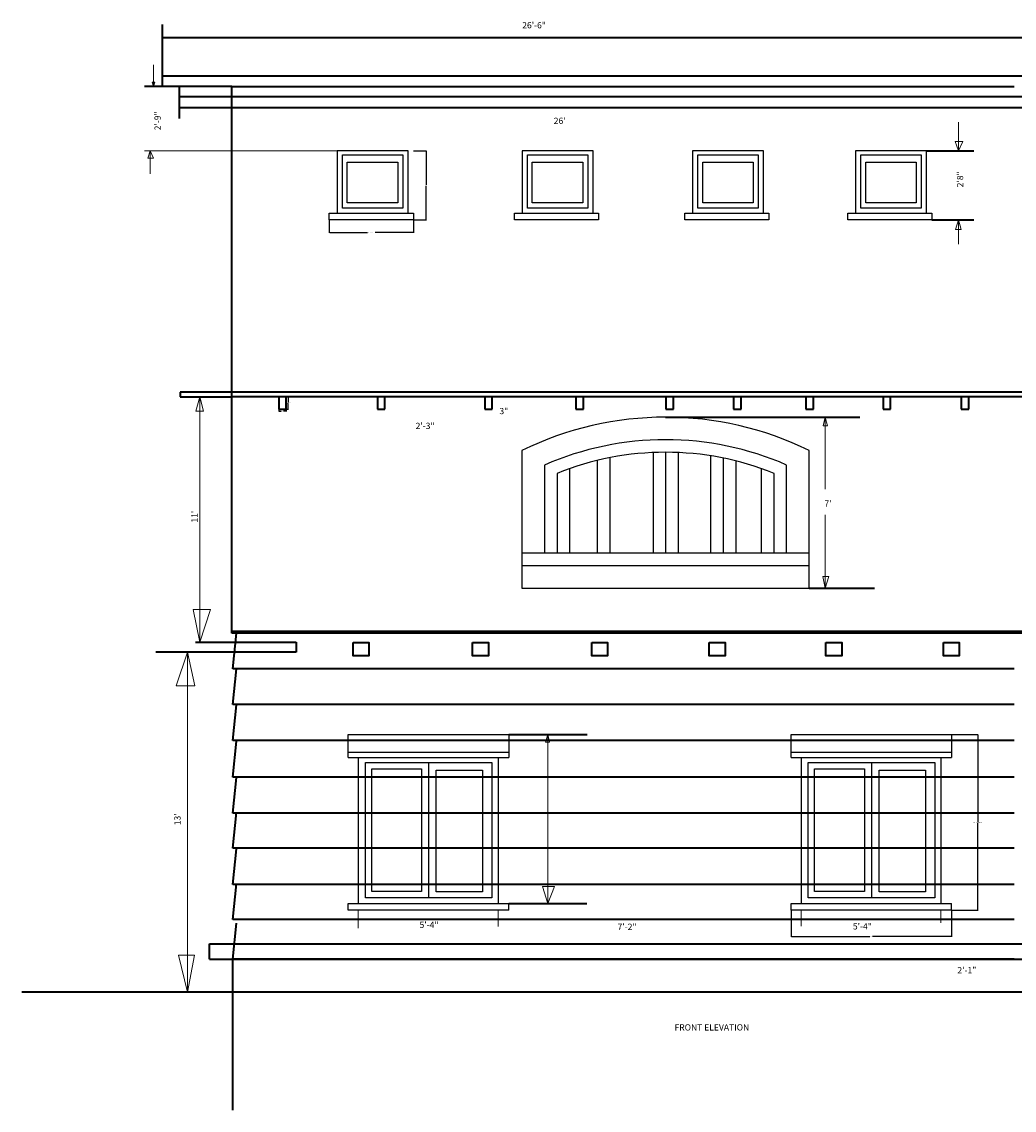
# Model space of a CAD drawing. Units: inches. Extents: x 2633 to 3277, y 1081 to 1518.
# Tile 1 of 2: x 2633 to 3029, y 1081 to 1515. Entities that reach past the tile are written whole.
import ezdxf

# ---------------------------------------------------------------- set-up
doc = ezdxf.new("R2010")
doc.units = ezdxf.units.IN
for name, color, linetype, lineweight in [('A-ANNO-DIMS', 2, 'Continuous', 18), ('A-ANNO-TEXT', 7, 'Continuous', 18), ('A-ELEV', 7, 'Continuous', 35), ('A-GLAZ', 4, 'Continuous', 25)]:
    doc.layers.add(name, color=color, linetype=linetype, lineweight=lineweight)
doc.styles.get("Standard").update_dxf_attribs({"font": 'arial.ttf'})
doc.dimstyles.get("Standard").update_dxf_attribs({"dimtxt": 0.18, "dimasz": 0.18, "dimexe": 0.18, "dimexo": 0.0625, "dimgap": 0.09, "dimtad": 0, "dimtih": 1, "dimtoh": 1, "dimdec": 4, "dimzin": 0, "dimdsep": 46, "dimtxsty": 'Standard', "dimcen": 0.09, "dimadec": 0, "dimazin": 0, "dimtfac": 1, "dimtdec": 4, "dimtofl": 0, "dimtmove": 0, "dimatfit": 3, "dimfxl": 1, "dimtolj": 1, "dimtzin": 0, "dimarcsym": 0})

# ---------------------------------------------------------------- blocks, each defined once
blk = doc.blocks.new('WIN-SMALL')
for points in [[(2758.75, 1438.68), (2787.06, 1438.68), (2787.06, 1463.6), (2758.75, 1463.6)], [(2760.89, 1461.89), (2784.92, 1461.89), (2784.92, 1440.71), (2760.89, 1440.71)], [(2762.78, 1458.97), (2782.94, 1458.97), (2782.94, 1442.85), (2762.78, 1442.85)], [(2755.63, 1438.68), (2789.18, 1438.68), (2789.18, 1436.03), (2755.63, 1436.03)]]:
    blk.add_lwpolyline(points, close=True)
blk = doc.blocks.new('WIN-1600-DBL')
for p, q in [((2763.18, 1221.7), (2763.18, 1230.77)), ((2763.18, 1230.77), (2827.18, 1230.77)), ((2827.18, 1230.77), (2827.18, 1221.7)), ((2763.18, 1223.71), (2827.18, 1223.77)), ((2763.18, 1221.7), (2827.18, 1221.7)), ((2767.18, 1221.7), (2767.18, 1163.47)), ((2822.92, 1221.7), (2822.92, 1163.47)), ((2795.24, 1219.61), (2795.24, 1165.66)), ((2763.18, 1160.77), (2763.18, 1163.47)), ((2763.18, 1163.47), (2827.18, 1163.47)), ((2827.18, 1160.77), (2827.18, 1163.47)), ((2827.18, 1160.77), (2763.18, 1160.77))]:
    blk.add_line(p, q)
for points in [[(2770, 1219.61), (2820.48, 1219.61), (2820.48, 1165.66), (2770, 1165.66)], [(2772.55, 1217.06), (2792.42, 1217.06), (2792.42, 1168.21), (2772.55, 1168.21)], [(2798.27, 1216.53), (2816.76, 1216.53), (2816.76, 1168.1), (2798.27, 1168.1)]]:
    blk.add_lwpolyline(points, close=True)
blk = doc.blocks.new('CORBEL-A')
for p, q in [((0, 4.96), (0, 0)), ((3, 0), (3, 4.96)), ((0, 0), (3, 0))]:
    blk.add_line(p, q)
blk = doc.blocks.new('*D6')
at = {"layer": 'A-ANNO-DIMS', "color": 0, "lineweight": -2, "transparency": 16777216}
for p, q in [((2755.63, 1435.97), (2755.63, 1430.82)), ((2789.18, 1435.97), (2789.18, 1430.82)), ((2755.81, 1431), (2770.84, 1431)), ((2789, 1431), (2773.97, 1431))]:
    blk.add_line(p, q, dxfattribs=at)
at = {"layer": 'A-ANNO-DIMS', "color": 0, "transparency": 16777216}
for points in [[(2755.81, 1431.03), (2755.81, 1430.97), (2755.63, 1431)], [(2789, 1431.03), (2789, 1430.97), (2789.18, 1431)]]:
    blk.add_solid(points, dxfattribs=at)
at = {"layer": 'Defpoints', "color": 0, "transparency": 16777216}
for p in [(2755.63, 1436.03), (2789.18, 1436.03), (2789.18, 1431)]:
    blk.add_point(p, dxfattribs=at)
at = {"layer": 'A-ANNO-DIMS', "color": 0, "transparency": 16777216, "insert": (2772.4, 1431), "char_height": 0.18, "attachment_point": 5}
blk.add_mtext('\\A1;SMALL WINDOW 34 TYP.', dxfattribs=at)
blk = doc.blocks.new('*D7')
at = {"layer": 'A-ANNO-DIMS', "color": 0, "lineweight": -2, "transparency": 16777216}
for p, q in [((2789.24, 1463.6), (2794.39, 1463.6)), ((2794.21, 1463.42), (2794.21, 1450)), ((2794.21, 1436.21), (2794.21, 1449.64)), ((2789.24, 1436.03), (2794.39, 1436.03))]:
    blk.add_line(p, q, dxfattribs=at)
at = {"layer": 'A-ANNO-DIMS', "color": 0, "transparency": 16777216}
for points in [[(2794.18, 1463.42), (2794.24, 1463.42), (2794.21, 1463.6)], [(2794.18, 1436.21), (2794.24, 1436.21), (2794.21, 1436.03)]]:
    blk.add_solid(points, dxfattribs=at)
at = {"layer": 'Defpoints', "color": 0, "transparency": 16777216}
for p in [(2789.18, 1463.6), (2794.21, 1463.6), (2789.18, 1436.03)]:
    blk.add_point(p, dxfattribs=at)
at = {"layer": 'A-ANNO-DIMS', "color": 0, "transparency": 16777216, "insert": (2794.21, 1449.82), "char_height": 0.18, "attachment_point": 5}
blk.add_mtext('\\A1;28 TYP.', dxfattribs=at)
blk = doc.blocks.new('*D8')
at = {"layer": 'A-ANNO-DIMS', "color": 0, "lineweight": -2, "transparency": 16777216}
for p, q in [((3003.8, 1230.77), (3014.41, 1230.77)), ((3014.23, 1230.59), (3014.23, 1195.96)), ((3014.23, 1160.95), (3014.23, 1195.59)), ((3003.8, 1160.77), (3014.41, 1160.77))]:
    blk.add_line(p, q, dxfattribs=at)
at = {"layer": 'A-ANNO-DIMS', "color": 0, "transparency": 16777216}
for points in [[(3014.2, 1230.59), (3014.26, 1230.59), (3014.23, 1230.77)], [(3014.2, 1160.95), (3014.26, 1160.95), (3014.23, 1160.77)]]:
    blk.add_solid(points, dxfattribs=at)
at = {"layer": 'Defpoints', "color": 0, "transparency": 16777216}
for p in [(3003.73, 1230.77), (3014.23, 1230.77), (3003.73, 1160.77)]:
    blk.add_point(p, dxfattribs=at)
at = {"layer": 'A-ANNO-DIMS', "color": 0, "transparency": 16777216, "insert": (3014.23, 1195.77), "char_height": 0.18, "attachment_point": 5}
blk.add_mtext('\\A1;DOUBLE WINDOW 1600 70 TYP.', dxfattribs=at)
blk = doc.blocks.new('*D9')
at = {"layer": 'A-ANNO-DIMS', "color": 0, "lineweight": -2, "transparency": 16777216}
for p, q in [((2939.73, 1160.71), (2939.73, 1150.09)), ((3003.73, 1160.71), (3003.73, 1150.09)), ((2939.91, 1150.27), (2971.21, 1150.27)), ((3003.55, 1150.27), (2972.26, 1150.27))]:
    blk.add_line(p, q, dxfattribs=at)
at = {"layer": 'A-ANNO-DIMS', "color": 0, "transparency": 16777216}
for points in [[(2939.91, 1150.3), (2939.91, 1150.24), (2939.73, 1150.27)], [(3003.55, 1150.3), (3003.55, 1150.24), (3003.73, 1150.27)]]:
    blk.add_solid(points, dxfattribs=at)
at = {"layer": 'Defpoints', "color": 0, "transparency": 16777216}
for p in [(2939.73, 1160.77), (3003.73, 1160.77), (3003.73, 1150.27)]:
    blk.add_point(p, dxfattribs=at)
at = {"layer": 'A-ANNO-DIMS', "color": 0, "transparency": 16777216, "insert": (2971.73, 1150.27), "char_height": 0.18, "attachment_point": 5}
blk.add_mtext('\\A1;64 TYP.', dxfattribs=at)
blk = doc.blocks.new('*D12')
at = {"layer": 'A-ANNO-DIMS', "color": 0, "lineweight": -2, "transparency": 16777216}
for p, q in [((2738.5, 1365.48), (2739.37, 1365.48)), ((2739.19, 1365.3), (2739.19, 1363.18)), ((2738.5, 1360.52), (2739.37, 1360.52)), ((2739.19, 1360.7), (2739.19, 1362.81))]:
    blk.add_line(p, q, dxfattribs=at)
at = {"layer": 'A-ANNO-DIMS', "color": 0, "transparency": 16777216}
for points in [[(2739.16, 1365.3), (2739.22, 1365.3), (2739.19, 1365.48)], [(2739.16, 1360.7), (2739.22, 1360.7), (2739.19, 1360.52)]]:
    blk.add_solid(points, dxfattribs=at)
at = {"layer": 'Defpoints', "color": 0, "transparency": 16777216}
for p in [(2738.44, 1365.48), (2739.19, 1365.48), (2738.44, 1360.52)]:
    blk.add_point(p, dxfattribs=at)
at = {"layer": 'A-ANNO-DIMS', "color": 0, "transparency": 16777216, "insert": (2739.19, 1363), "char_height": 0.18, "attachment_point": 5}
blk.add_mtext('\\A1;CORBEL A 5 TYP.', dxfattribs=at)
blk = doc.blocks.new('*D13')
at = {"layer": 'A-ANNO-DIMS', "color": 0, "lineweight": -2, "transparency": 16777216}
for p, q in [((2735.44, 1360.45), (2735.44, 1359.59)), ((2735.62, 1359.77), (2736.48, 1359.77)), ((2738.26, 1359.77), (2737.4, 1359.77)), ((2738.44, 1360.45), (2738.44, 1359.59))]:
    blk.add_line(p, q, dxfattribs=at)
at = {"layer": 'A-ANNO-DIMS', "color": 0, "transparency": 16777216}
for points in [[(2735.62, 1359.8), (2735.62, 1359.74), (2735.44, 1359.77)], [(2738.26, 1359.8), (2738.26, 1359.74), (2738.44, 1359.77)]]:
    blk.add_solid(points, dxfattribs=at)
at = {"layer": 'Defpoints', "color": 0, "transparency": 16777216}
for p in [(2735.44, 1360.52), (2738.44, 1360.52), (2738.44, 1359.77)]:
    blk.add_point(p, dxfattribs=at)
at = {"layer": 'A-ANNO-DIMS', "color": 0, "transparency": 16777216, "insert": (2736.94, 1359.77), "char_height": 0.18, "attachment_point": 5}
blk.add_mtext('\\A1;3 TYP.', dxfattribs=at)

msp = doc.modelspace()

# ---------------------------------------------------------------- linework, layer by layer
at = {"layer": 'A-ANNO-DIMS'}
for p, q in [((2685.55, 1489.27), (2685.55, 1497.82)), ((2685.55, 1489.27), (2685.05, 1490.87)), ((2685.05, 1490.87), (2686.02, 1490.87)), ((2686.02, 1490.87), (2685.55, 1489.27)), ((3006.52, 1463.6), (3006.52, 1474.98)), ((3006.52, 1463.6), (3005.21, 1467.22)), ((3005.21, 1467.22), (3008.18, 1467.22)), ((3008.18, 1467.22), (3006.52, 1463.6)), ((2684.17, 1463.6), (2682, 1463.6)), ((2684.17, 1463.6), (2683.31, 1460.56)), ((2758.75, 1463.6), (2684.17, 1463.6)), ((2684.17, 1463.6), (2684.17, 1454.36)), ((2685.55, 1460.56), (2684.17, 1463.6)), ((2683.31, 1460.56), (2685.55, 1460.56)), ((3006.52, 1436.03), (3005.33, 1432.15)), ((3006.52, 1436.03), (3006.52, 1426.33)), ((3007.59, 1432.15), (3006.52, 1436.03)), ((3005.33, 1432.15), (3007.59, 1432.15)), ((2704.03, 1365.48), (2702.38, 1359.8)), ((2704.03, 1365.48), (2704.03, 1267.58)), ((2705.46, 1359.8), (2704.03, 1365.48)), ((2702.38, 1359.8), (2705.46, 1359.8)), ((2953.34, 1357.35), (2952.57, 1353.88)), ((2953.34, 1357.35), (2953.34, 1328.63)), ((2954.23, 1353.88), (2953.34, 1357.35)), ((2952.57, 1353.88), (2954.23, 1353.88)), ((2953.34, 1318.37), (2953.34, 1289.2)), ((2953.34, 1289.2), (2952.42, 1293.75)), ((2952.42, 1293.75), (2954.75, 1293.75)), ((2954.75, 1293.75), (2953.34, 1289.2)), ((2704.03, 1267.58), (2701.36, 1280.64)), ((2701.36, 1280.64), (2708.25, 1280.64)), ((2708.25, 1280.64), (2704.03, 1267.58)), ((2699.04, 1263.58), (2694.62, 1250.15)), ((2699.04, 1263.58), (2699.04, 1128.1)), ((2702.02, 1250.15), (2699.04, 1263.58)), ((2694.62, 1250.15), (2702.02, 1250.15)), ((2842.72, 1230.77), (2841.86, 1227.77)), ((2842.72, 1163.47), (2842.72, 1230.77)), ((2843.41, 1227.77), (2842.72, 1230.77)), ((2841.86, 1227.77), (2843.41, 1227.77)), ((2842.72, 1163.47), (2840.59, 1170.21)), ((2840.59, 1170.21), (2845.42, 1170.21)), ((2845.42, 1170.21), (2842.72, 1163.47)), ((2767.18, 1160.77), (2767.18, 1153.52)), ((2822.92, 1160.77), (2822.92, 1154.28)), ((2943.73, 1160.77), (2943.73, 1154.35)), ((2999.47, 1160.77), (2999.47, 1155.65)), ((2699.04, 1128.1), (2695.5, 1142.8)), ((2695.5, 1142.8), (2701.93, 1142.8)), ((2701.93, 1142.8), (2699.04, 1128.1))]:
    msp.add_line(p, q, dxfattribs=at)
at = {"layer": 'A-ELEV'}
for p, q in [((2689.1, 1493.43), (2689.1, 1513.93)), ((2689.1, 1508.71), (3038.3, 1508.71)), ((2689.1, 1489.27), (2689.1, 1493.43)), ((2689.1, 1493.43), (3038.3, 1493.43)), ((2689.1, 1489.27), (2682, 1489.27)), ((2716.73, 1489.27), (2689.1, 1489.27)), ((2695.73, 1489.27), (2695.73, 1485.17)), ((2716.73, 1403.27), (2716.73, 1489.27)), ((2716.73, 1489.27), (3028.73, 1489.27)), ((2695.73, 1485.17), (3034.63, 1485.17)), ((2695.73, 1485.17), (2695.73, 1476.45)), ((2695.73, 1480.81), (3034.63, 1480.81)), ((2993.79, 1463.6), (3012.64, 1463.6)), ((2995.9, 1436.03), (3012.64, 1436.03)), ((2716.73, 1271.27), (2716.73, 1403.27)), ((2716.73, 1367.27), (2696.18, 1367.27)), ((2696.18, 1367.27), (2696.18, 1365.48)), ((2852.9, 1367.27), (2716.73, 1367.27)), ((3213.81, 1367.27), (2852.9, 1367.27)), ((2696.18, 1365.48), (2716.73, 1365.48)), ((2840.38, 1365.48), (2716.73, 1365.48)), ((3199.77, 1365.48), (2840.38, 1365.48)), ((2916.84, 1365.48), (2916.84, 1360.52)), ((2916.84, 1365.48), (2916.84, 1360.52)), ((2916.84, 1365.48), (2916.84, 1360.52)), ((2919.84, 1360.52), (2919.84, 1365.48)), ((2919.84, 1360.52), (2919.84, 1365.48)), ((2919.84, 1360.52), (2919.84, 1365.48)), ((2916.84, 1360.52), (2919.84, 1360.52)), ((2916.84, 1360.52), (2919.84, 1360.52)), ((2916.84, 1360.52), (2919.84, 1360.52)), ((2889.71, 1357.35), (2967.21, 1357.35)), ((2946.97, 1289.2), (2972.98, 1289.2)), ((2888.3, 1271.83), (2716.73, 1271.83)), ((3209.71, 1271.83), (2888.3, 1271.83)), ((2888.3, 1271.83), (2888.3, 1271.27)), ((2702.3, 1267.58), (2742.42, 1267.58)), ((2888.3, 1271.27), (2716.73, 1271.27)), ((2717.1, 1257), (2718.63, 1271.27)), ((2742.42, 1267.58), (2742.42, 1263.58)), ((3197.44, 1271.27), (2888.3, 1271.27)), ((2702.3, 1263.58), (2686.43, 1263.58)), ((2742.42, 1263.58), (2702.3, 1263.58)), ((2717.1, 1242.79), (2718.63, 1257.05)), ((3028.73, 1257), (2717.1, 1257)), ((3028.73, 1242.79), (2717.1, 1242.79)), ((2717.1, 1228.4), (2718.63, 1242.66)), ((3028.73, 1228.4), (2717.1, 1228.4)), ((2827.18, 1230.77), (2858.42, 1230.77)), ((2717.1, 1213.84), (2718.63, 1228.1)), ((3028.73, 1213.84), (2717.1, 1213.84)), ((2717.1, 1199.45), (2718.63, 1213.71)), ((2717.1, 1185.43), (2718.63, 1199.69)), ((3028.73, 1199.45), (2717.1, 1199.45)), ((3028.73, 1185.43), (2717.1, 1185.43)), ((2717.1, 1170.99), (2718.63, 1185.25)), ((2717.1, 1156.97), (2718.63, 1171.23)), ((3028.73, 1170.99), (2717.1, 1170.99)), ((2827.18, 1163.47), (2858.25, 1163.47)), ((3028.73, 1156.97), (2717.1, 1156.97)), ((2717.1, 1141.27), (2718.63, 1155.53)), ((2707.86, 1141.27), (2707.86, 1147.27)), ((2707.86, 1147.27), (3211.86, 1147.27)), ((2707.86, 1141.27), (3211.86, 1141.27)), ((2717.04, 1141.27), (2717.04, 1080.98)), ((3028.73, 1141.27), (2717.1, 1141.27)), ((3032.99, 1128.1), (2633.01, 1128.1))]:
    msp.add_line(p, q, dxfattribs=at)
for points in [[(2765.13, 1267.47), (2771.4, 1267.47), (2771.4, 1262.19), (2765.13, 1262.19)], [(2812.78, 1267.47), (2819.05, 1267.47), (2819.05, 1262.19), (2812.78, 1262.19)], [(2860.27, 1267.47), (2866.54, 1267.47), (2866.54, 1262.19), (2860.27, 1262.19)], [(2907.16, 1267.47), (2913.43, 1267.47), (2913.43, 1262.19), (2907.16, 1262.19)], [(2953.66, 1267.47), (2959.93, 1267.47), (2959.93, 1262.19), (2953.66, 1262.19)], [(3000.56, 1267.47), (3006.83, 1267.47), (3006.83, 1262.19), (3000.56, 1262.19)]]:
    msp.add_lwpolyline(points, close=True, dxfattribs=at)
at = {"layer": 'A-GLAZ'}
for p, q in [((2832.44, 1344), (2832.44, 1289.2)), ((2867.45, 1341.19), (2867.45, 1303.2)), ((2884.71, 1343.24), (2884.71, 1303.2)), ((2889.71, 1343.35), (2889.71, 1303.2)), ((2894.71, 1343.24), (2894.71, 1303.2)), ((2907.68, 1341.94), (2907.68, 1303.2)), ((2946.97, 1289.2), (2946.97, 1344)), ((2841.44, 1338.26), (2841.44, 1303.2)), ((2862.45, 1340.09), (2862.45, 1303.2)), ((2912.68, 1341.04), (2912.68, 1303.2)), ((2917.68, 1339.91), (2917.68, 1303.2)), ((2937.97, 1303.2), (2937.97, 1338.26)), ((2846.44, 1334.94), (2846.44, 1303.2)), ((2851.44, 1336.83), (2851.44, 1303.2)), ((2927.97, 1303.2), (2927.97, 1336.83)), ((2932.97, 1303.2), (2932.97, 1334.94)), ((2832.44, 1303.2), (2946.97, 1303.2)), ((2832.44, 1298.2), (2946.97, 1298.2)), ((2832.44, 1289.2), (2946.97, 1289.2))]:
    msp.add_line(p, q, dxfattribs=at)
for radius, start, end in [(129.5, 63.7561, 116.2439), (120.5, 66.3885, 113.6115), (115.5, 68.0015, 111.9985)]:
    msp.add_arc((2889.71, 1227.85), radius, start, end, dxfattribs=at)

# ---------------------------------------------------------------- block references
at = {"layer": 'A-ELEV'}
for p in [(2735.44, 1360.52), (2774.79, 1360.52), (2817.62, 1360.52), (2853.95, 1360.52), (2889.84, 1360.52), (2945.64, 1360.52), (2976.43, 1360.52), (3007.57, 1360.52)]:
    msp.add_blockref('CORBEL-A', p, dxfattribs=at)
at = {"layer": 'A-GLAZ'}
for name, p in [('WIN-SMALL', (0, 0)), ('WIN-SMALL', (73.8, 0)), ('WIN-SMALL', (141.74, 0)), ('WIN-SMALL', (206.73, 0)), ('WIN-1600-DBL', (0, 0)), ('WIN-1600-DBL', (176.55, 0))]:
    msp.add_blockref(name, p, dxfattribs=at)

# ---------------------------------------------------------------- texts
at = {"layer": 'A-ANNO-TEXT', "char_height": 2.5, "attachment_point": 1}
for s, width, insert in [('26\'-6"', 11.5627, (2832.55, 1514.89)), ("26'", 9.8582, (2845.12, 1476.78)), ('3"', 5.0263, (2823.48, 1361.04)), ('2\'-3"', 14.2854, (2790.05, 1355.13)), ("7'", 7.8526, (2953.06, 1324.19)), ('5\'-4"', 12.5637, (2791.62, 1156.15)), ('7\'-2"', 16.8387, (2870.58, 1155.39)), ('5\'-4"', 12.0401, (2964.4, 1155.55)), ('2\'-1"', 16.1936, (3006.09, 1138.09)), ('FRONT ELEVATION', 167.4705, (2893.28, 1115.27))]:
    msp.add_mtext_dynamic_manual_height_columns(s, width=width, gutter_width=12.5, heights=[0], dxfattribs=dict(at, insert=insert))
at = {"layer": 'A-ANNO-TEXT', "char_height": 2.5, "attachment_point": 1, "rotation": 90}
for s, width, insert in [('2\'-9"', 7.2606, (2685.92, 1471.74)), ('2\'8"', 9.6466, (3005.91, 1449)), ("11'", 10.87, (2700.6, 1315.3)), ("13'", 12.8631, (2693.82, 1194.62))]:
    msp.add_mtext_dynamic_manual_height_columns(s, width=width, gutter_width=12.5, heights=[0], dxfattribs=dict(at, insert=insert))

# ---------------------------------------------------------------- dimensions: what is measured, and where the dimension line sits
at = {"layer": 'A-ANNO-DIMS'}
for base, p1, p2, text, picture, middle in [((2794.21, 1463.6), (2789.18, 1436.03), (2789.18, 1463.6), '<> TYP.', '*D7', (2794.21, 1449.82)), ((2739.19, 1365.48), (2738.44, 1360.52), (2738.44, 1365.48), 'CORBEL A <> TYP.', '*D12', (2739.19, 1363)), ((3014.23, 1230.77), (3003.73, 1160.77), (3003.73, 1230.77), 'DOUBLE WINDOW 1600 <> TYP.', '*D8', (3014.23, 1195.77))]:
    dim = msp.add_linear_dim(base=base, p1=p1, p2=p2, angle=90, text=text, dimstyle='Standard', override={"dimdec": 0, "dimlfac": 1, "dimrnd": 0, "dimzin": 0, "dimdsep": 46, "dimlunit": 2}, dxfattribs=at)
    dim.commit()
    dim.dimension.update_dxf_attribs({"geometry": picture, "text_midpoint": middle})
for base, p1, p2, text, picture, middle in [((2789.18, 1431), (2755.63, 1436.03), (2789.18, 1436.03), 'SMALL WINDOW <> TYP.', '*D6', (2772.4, 1431)), ((2738.44, 1359.77), (2735.44, 1360.52), (2738.44, 1360.52), '<> TYP.', '*D13', (2736.94, 1359.77)), ((3003.73, 1150.27), (2939.73, 1160.77), (3003.73, 1160.77), '<> TYP.', '*D9', (2971.73, 1150.27))]:
    dim = msp.add_linear_dim(base=base, p1=p1, p2=p2, text=text, dimstyle='Standard', override={"dimdec": 0, "dimlfac": 1, "dimrnd": 0, "dimzin": 0, "dimdsep": 46, "dimlunit": 2}, dxfattribs=at)
    dim.commit()
    dim.dimension.update_dxf_attribs({"geometry": picture, "text_midpoint": middle})

doc.saveas('drawing.dxf')
